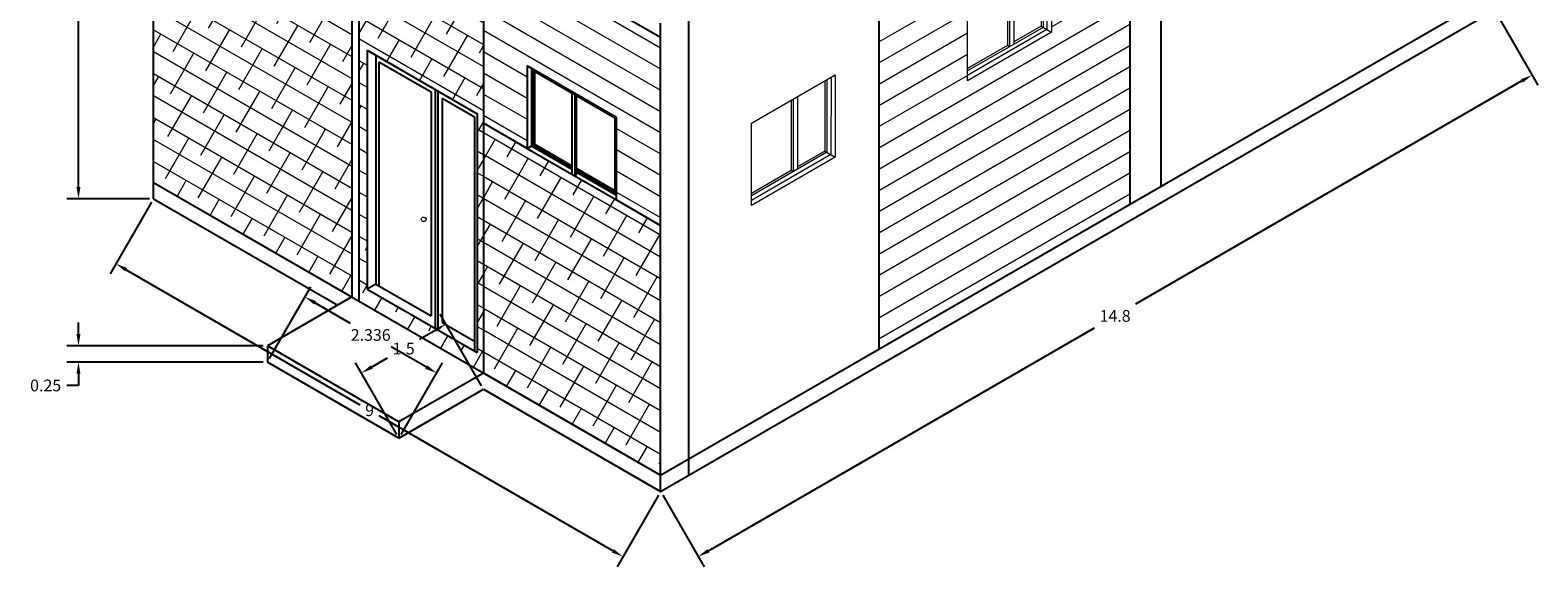
# Model space of a CAD drawing. Units: metres. Extents: x 14054 to 28215, y 4175 to 8383.
# Tile 1 of 6: x 14054 to 14077, y 4175 to 4183. Entities that reach past the tile are written whole.
import ezdxf

# ---------------------------------------------------------------- set-up
doc = ezdxf.new("R2010")
doc.units = ezdxf.units.M
for name, color, linetype, lineweight in [('A-ANNO-DIMS', 2, 'Continuous', 18), ('A-ELEV-ISOM', 7, 'Continuous', 25), ('A-FURN', 8, 'Continuous', 13), ('A-GLAZ', 4, 'Continuous', 18), ('A-WALL-PATT', 8, 'Continuous', 13)]:
    doc.layers.add(name, color=color, linetype=linetype, lineweight=lineweight)
doc.styles.get("Standard").update_dxf_attribs({"font": 'arial.ttf'})
doc.dimstyles.get("Standard").update_dxf_attribs({"dimtxt": 0.18, "dimasz": 0.18, "dimexe": 0.18, "dimexo": 0.0625, "dimgap": 0.09, "dimtad": 0, "dimtih": 1, "dimtoh": 1, "dimdec": 4, "dimzin": 0, "dimdsep": 46, "dimtxsty": 'Standard', "dimcen": 0.09, "dimadec": 0, "dimazin": 0, "dimtfac": 1, "dimtdec": 4, "dimtofl": 0, "dimtmove": 0, "dimatfit": 3, "dimfxl": 1, "dimtolj": 1, "dimtzin": 0, "dimarcsym": 0})

# ---------------------------------------------------------------- blocks, each defined once
blk = doc.blocks.new('WINDOW 1')
for p, q in [((14073.717, 4186.789), (14075.449, 4187.789)), ((14075.233, 4187.664), (14075.233, 4186.214)), ((14075.276, 4187.689), (14075.276, 4186.189)), ((14075.365, 4187.74), (14075.356, 4186.143)), ((14075.449, 4187.789), (14075.449, 4186.089)), ((14074.67, 4187.34), (14074.67, 4185.84)), ((14074.54, 4187.264), (14074.54, 4185.814)), ((14074.583, 4187.289), (14074.583, 4185.789)), ((14073.717, 4185.089), (14073.717, 4186.789)), ((14075.276, 4186.189), (14073.717, 4185.289)), ((14075.356, 4186.143), (14073.717, 4185.197)), ((14075.449, 4186.089), (14073.717, 4185.089)), ((14075.233, 4186.214), (14074.67, 4185.889)), ((14075.233, 4186.214), (14075.449, 4186.089)), ((14074.54, 4185.814), (14073.717, 4185.339)), ((14074.583, 4185.789), (14074.54, 4185.814))]:
    blk.add_line(p, q)
blk = doc.blocks.new('*D10')
at = {"layer": 'A-ANNO-DIMS', "color": 0, "lineweight": -2, "transparency": 16777216}
for p, q in [((14055.747, 4180.437), (14055.111, 4179.335)), ((14055.357, 4179.401), (14058.949, 4177.327)), ((14062.839, 4175.081), (14059.247, 4177.155)), ((14063.541, 4175.937), (14062.905, 4174.835))]:
    blk.add_line(p, q, dxfattribs=at)
at = {"layer": 'A-ANNO-DIMS', "color": 0, "transparency": 16777216}
for points in [[(14055.372, 4179.427), (14055.342, 4179.375), (14055.201, 4179.491)], [(14062.854, 4175.107), (14062.824, 4175.055), (14062.995, 4174.991)]]:
    blk.add_solid(points, dxfattribs=at)
at = {"layer": 'Defpoints', "color": 0, "transparency": 16777216}
for p in [(14055.778, 4180.491), (14055.201, 4179.491), (14063.573, 4175.991)]:
    blk.add_point(p, dxfattribs=at)
at = {"layer": 'A-ANNO-DIMS', "color": 0, "transparency": 16777216, "insert": (14059.098, 4177.241), "char_height": 0.18, "attachment_point": 5}
blk.add_mtext('\\A1;9', dxfattribs=at)
blk = doc.blocks.new('*D11')
at = {"layer": 'A-ANNO-DIMS', "color": 0, "lineweight": -2, "transparency": 16777216}
for p, q in [((14076.421, 4183.337), (14077.057, 4182.235)), ((14076.812, 4182.301), (14070.874, 4178.873)), ((14064.306, 4175.081), (14070.244, 4178.509)), ((14063.604, 4175.937), (14064.24, 4174.835))]:
    blk.add_line(p, q, dxfattribs=at)
at = {"layer": 'A-ANNO-DIMS', "color": 0, "transparency": 16777216}
for points in [[(14076.797, 4182.327), (14076.827, 4182.275), (14076.967, 4182.391)], [(14064.291, 4175.107), (14064.321, 4175.055), (14064.15, 4174.991)]]:
    blk.add_solid(points, dxfattribs=at)
at = {"layer": 'Defpoints', "color": 0, "transparency": 16777216}
for p in [(14076.39, 4183.391), (14063.573, 4175.991), (14064.15, 4174.991)]:
    blk.add_point(p, dxfattribs=at)
at = {"layer": 'A-ANNO-DIMS', "color": 0, "transparency": 16777216, "insert": (14070.559, 4178.691), "char_height": 0.18, "attachment_point": 5}
blk.add_mtext('\\A1;14.8', dxfattribs=at)
blk = doc.blocks.new('*D12')
at = {"layer": 'A-ANNO-DIMS', "color": 0, "lineweight": -2, "transparency": 16777216}
for p, q in [((14055.716, 4190.691), (14054.443, 4190.691)), ((14054.623, 4190.511), (14054.623, 4185.773)), ((14054.623, 4180.671), (14054.623, 4185.409)), ((14055.716, 4180.491), (14054.443, 4180.491))]:
    blk.add_line(p, q, dxfattribs=at)
at = {"layer": 'A-ANNO-DIMS', "color": 0, "transparency": 16777216}
for points in [[(14054.593, 4190.511), (14054.653, 4190.511), (14054.623, 4190.691)], [(14054.593, 4180.671), (14054.653, 4180.671), (14054.623, 4180.491)]]:
    blk.add_solid(points, dxfattribs=at)
at = {"layer": 'Defpoints', "color": 0, "transparency": 16777216}
for p in [(14054.623, 4190.691), (14055.778, 4190.691), (14055.778, 4180.491)]:
    blk.add_point(p, dxfattribs=at)
at = {"layer": 'A-ANNO-DIMS', "color": 0, "transparency": 16777216, "insert": (14054.623, 4185.591), "char_height": 0.18, "attachment_point": 5}
blk.add_mtext('\\A1;10.2', dxfattribs=at)
blk = doc.blocks.new('*D67')
at = {"layer": 'A-ANNO-DIMS', "color": 0, "lineweight": -2, "transparency": 16777216}
for p, q in [((14057.558, 4178.036), (14058.195, 4179.138)), ((14058.261, 4178.892), (14058.801, 4178.58)), ((14059.972, 4177.904), (14059.431, 4178.216)), ((14059.582, 4176.868), (14060.218, 4177.97))]:
    blk.add_line(p, q, dxfattribs=at)
at = {"layer": 'A-ANNO-DIMS', "color": 0, "transparency": 16777216}
for points in [[(14058.276, 4178.918), (14058.246, 4178.866), (14058.105, 4178.982)], [(14059.987, 4177.93), (14059.957, 4177.878), (14060.128, 4177.814)]]:
    blk.add_solid(points, dxfattribs=at)
at = {"layer": 'Defpoints', "color": 0, "transparency": 16777216}
for p in [(14057.527, 4177.982), (14060.128, 4177.814), (14059.55, 4176.814)]:
    blk.add_point(p, dxfattribs=at)
at = {"layer": 'A-ANNO-DIMS', "color": 0, "transparency": 16777216, "insert": (14059.116, 4178.398), "char_height": 0.18, "attachment_point": 5}
blk.add_mtext('\\A1;2.336', dxfattribs=at)
blk = doc.blocks.new('*D68')
at = {"layer": 'A-ANNO-DIMS', "color": 0, "lineweight": -2, "transparency": 16777216}
for p, q in [((14060.818, 4177.618), (14060.182, 4178.72)), ((14060.116, 4178.474), (14059.868, 4178.331)), ((14059.519, 4176.868), (14058.883, 4177.97)), ((14059.129, 4177.904), (14059.376, 4178.047))]:
    blk.add_line(p, q, dxfattribs=at)
at = {"layer": 'A-ANNO-DIMS', "color": 0, "transparency": 16777216}
for points in [[(14060.101, 4178.5), (14060.131, 4178.448), (14060.272, 4178.564)], [(14059.114, 4177.93), (14059.144, 4177.878), (14058.973, 4177.814)]]:
    blk.add_solid(points, dxfattribs=at)
at = {"layer": 'Defpoints', "color": 0, "transparency": 16777216}
for p in [(14060.272, 4178.564), (14060.849, 4177.564), (14059.55, 4176.814)]:
    blk.add_point(p, dxfattribs=at)
at = {"layer": 'A-ANNO-DIMS', "color": 0, "transparency": 16777216, "insert": (14059.622, 4178.189), "char_height": 0.18, "attachment_point": 5}
blk.add_mtext('\\A1;1.5', dxfattribs=at)
blk = doc.blocks.new('*D69')
at = {"layer": 'A-ANNO-DIMS', "color": 0, "lineweight": -2, "transparency": 16777216}
for p, q in [((14054.623, 4178.412), (14054.623, 4178.592)), ((14057.465, 4178.232), (14054.443, 4178.232)), ((14057.465, 4177.982), (14054.443, 4177.982)), ((14054.623, 4177.802), (14054.623, 4177.622)), ((14054.623, 4177.622), (14054.443, 4177.622))]:
    blk.add_line(p, q, dxfattribs=at)
at = {"layer": 'A-ANNO-DIMS', "color": 0, "transparency": 16777216}
for points in [[(14054.593, 4178.412), (14054.653, 4178.412), (14054.623, 4178.232)], [(14054.593, 4177.802), (14054.653, 4177.802), (14054.623, 4177.982)]]:
    blk.add_solid(points, dxfattribs=at)
at = {"layer": 'Defpoints', "color": 0, "transparency": 16777216}
for p in [(14057.527, 4178.232), (14054.623, 4177.982), (14057.527, 4177.982)]:
    blk.add_point(p, dxfattribs=at)
at = {"layer": 'A-ANNO-DIMS', "color": 0, "transparency": 16777216, "insert": (14054.119, 4177.622), "char_height": 0.18, "attachment_point": 5}
blk.add_mtext('\\A1;0.25', dxfattribs=at)

msp = doc.modelspace()

# ---------------------------------------------------------------- hatches: boundary and pattern name
at = {"layer": 'A-WALL-PATT'}
h = msp.add_hatch(dxfattribs=at)
h.set_pattern_fill('ANSI38', color=256, scale=0.092, angle=105)
h.paths.add_polyline_path([(14055.7785, 4187.4672), (14055.7785, 4180.7413), (14058.8262, 4178.9816), (14058.8262, 4185.7075)])
h.paths.add_polyline_path([(14058.0676, 4184.5273), (14058.0676, 4183.2595), (14056.6953, 4184.0519), (14056.6953, 4185.3196)], flags=16)
h.paths.add_polyline_path([(14056.7604, 4184.0895), (14056.7893, 4184.1061), (14056.7893, 4185.2436), (14058.0488, 4184.5164), (14058.0488, 4183.401), (14057.4455, 4183.7494), (14057.4455, 4183.6399), (14057.4272, 4183.6293), (14057.4272, 4184.8753), (14057.3815, 4184.9017), (14057.3815, 4183.7309)], flags=0)
h.paths.add_polyline_path([(14063.5727, 4180.0812), (14062.8942, 4180.4729), (14061.5218, 4181.2653), (14060.8587, 4181.6535), (14060.8401, 4177.8243), (14063.5727, 4176.2413)])
h.paths.add_polyline_path([(14060.8494, 4184.7636), (14060.9576, 4184.8261), (14058.9345, 4185.9941), (14058.9345, 4178.9191), (14060.8494, 4177.8136)])
h.paths.add_polyline_path([(14060.7529, 4181.7978), (14060.7529, 4181.7242), (14060.7529, 4178.127), (14059.0613, 4179.1036), (14059.0613, 4182.7744)], flags=16)
h.paths.add_polyline_path([(14059.2399, 4179.1538), (14059.2399, 4182.5977), (14060.0427, 4182.1342), (14060.0427, 4178.6903)], flags=0)
h.paths.add_polyline_path([(14060.215, 4182.0347), (14060.7096, 4181.7492), (14060.7096, 4178.3053), (14060.215, 4178.5908)], flags=0)
edge = h.paths.add_edge_path(flags=0)
edge.add_ellipse((14059.9307, 4180.1763), major_axis=(-0.0333, 0.0192), ratio=0.8810932, start_angle=0, end_angle=360)
h = msp.add_hatch(dxfattribs=at)
h.set_pattern_fill('ANSI31', color=256, scale=0.089, angle=165)
h.paths.add_polyline_path([(14070.7875, 4187.3567), (14066.9286, 4185.1288), (14066.9286, 4178.1788), (14070.7875, 4180.4067)])
h.paths.add_polyline_path([(14069.5808, 4184.3152), (14069.5808, 4183.05), (14068.2917, 4182.3057), (14068.2917, 4183.5709)], flags=16)
h.paths.add_polyline_path([(14069.4519, 4183.1244), (14069.0007, 4182.8639), (14069.0007, 4182.9011), (14069.4197, 4183.143)], flags=0)
h = msp.add_hatch(dxfattribs=at)
h.set_pattern_fill('ANSI31', color=256, scale=0.089, angle=105)
h.paths.add_polyline_path([(14063.5727, 4182.9672), (14060.8494, 4184.5395), (14060.8494, 4181.6535), (14061.5218, 4181.2653), (14061.5218, 4182.533), (14062.8942, 4181.7407), (14062.8942, 4180.4729), (14063.5727, 4180.0812)])

# ---------------------------------------------------------------- linework, layer by layer
at = {"layer": 'A-ELEV-ISOM'}
for p, q in [((14070.7875, 4190.3575), (14070.7875, 4180.4067)), ((14055.7785, 4180.4913), (14055.7785, 4187.6913)), ((14071.2638, 4187.6317), (14071.2638, 4180.6817)), ((14058.9345, 4185.9941), (14058.9345, 4178.9191)), ((14058.8262, 4185.9316), (14058.8262, 4178.9816)), ((14066.9286, 4185.1288), (14066.9286, 4178.1788)), ((14060.8494, 4184.7636), (14060.8494, 4177.8136)), ((14063.5727, 4182.9672), (14060.8494, 4184.5395)), ((14063.5727, 4176.2413), (14076.3899, 4183.6413)), ((14064.0057, 4176.2413), (14064.0057, 4183.4413)), ((14063.5727, 4175.9913), (14076.3899, 4183.3913)), ((14063.5727, 4175.9913), (14063.5727, 4183.1913)), ((14059.0613, 4182.7744), (14060.7529, 4181.7978)), ((14059.0613, 4182.7744), (14059.0613, 4179.1036)), ((14059.194, 4182.6978), (14059.194, 4179.1803)), ((14059.2399, 4182.5977), (14060.0427, 4182.1342)), ((14059.2399, 4182.5977), (14059.2399, 4179.1538)), ((14062.8942, 4181.7407), (14061.5218, 4182.533)), ((14061.5218, 4182.533), (14061.5218, 4181.2653)), ((14061.5869, 4182.4954), (14061.5869, 4181.3029)), ((14061.6158, 4182.457), (14061.6158, 4181.3195)), ((14062.8754, 4181.7298), (14061.6158, 4182.457)), ((14061.635, 4182.446), (14061.635, 4181.3306)), ((14060.0427, 4182.1342), (14060.0427, 4178.6903)), ((14060.1077, 4182.1703), (14060.1077, 4178.4995)), ((14060.1465, 4182.1479), (14060.1465, 4178.4771)), ((14062.208, 4182.1151), (14062.208, 4180.8691)), ((14062.2537, 4182.0887), (14062.2537, 4180.8427)), ((14062.272, 4182.0781), (14062.272, 4180.8533)), ((14060.215, 4182.0347), (14060.215, 4178.5908)), ((14060.215, 4182.0347), (14060.7096, 4181.7492)), ((14060.7096, 4181.7492), (14060.7096, 4178.152)), ((14060.7529, 4181.7978), (14060.7529, 4181.7242)), ((14060.7529, 4181.7242), (14060.7529, 4178.127)), ((14061.5218, 4181.2653), (14060.8494, 4181.6535)), ((14062.8754, 4180.6144), (14062.8754, 4181.7298)), ((14062.8942, 4180.4729), (14062.8942, 4181.7407)), ((14061.5218, 4181.2653), (14061.635, 4181.3306)), ((14061.5218, 4181.2653), (14062.8942, 4180.4729)), ((14061.5869, 4181.3029), (14062.208, 4180.9443)), ((14061.6158, 4181.3195), (14062.208, 4180.9777)), ((14061.635, 4181.3306), (14062.208, 4180.9997)), ((14062.272, 4180.9628), (14062.8754, 4180.6144)), ((14062.272, 4180.9407), (14062.8942, 4180.5815)), ((14062.272, 4180.9073), (14062.8942, 4180.5481)), ((14055.7785, 4180.7413), (14063.5727, 4176.2413)), ((14055.7785, 4180.7413), (14058.8262, 4178.9816)), ((14062.2537, 4180.8427), (14062.272, 4180.8533)), ((14055.7785, 4180.4913), (14058.6097, 4178.8566)), ((14062.8942, 4180.4729), (14063.5727, 4180.0812)), ((14059.194, 4179.1803), (14059.0613, 4179.1036)), ((14059.0613, 4179.1036), (14060.7529, 4178.127)), ((14059.194, 4179.1803), (14060.0427, 4178.6903)), ((14058.8262, 4178.9816), (14057.5272, 4178.2316)), ((14060.215, 4178.5908), (14060.7096, 4178.3053)), ((14059.5503, 4177.0636), (14057.5272, 4178.2316)), ((14057.5272, 4178.2316), (14057.5272, 4177.9816)), ((14059.5503, 4176.8136), (14057.5272, 4177.9816)), ((14060.8494, 4177.8136), (14059.5503, 4177.0636)), ((14060.8308, 4177.8243), (14063.5727, 4176.2413)), ((14059.5503, 4176.8136), (14060.8494, 4177.5636)), ((14060.8494, 4177.5636), (14063.5727, 4175.9913)), ((14059.5503, 4177.0636), (14059.5503, 4176.8136))]:
    msp.add_line(p, q, dxfattribs=at)
at = {"layer": 'A-FURN'}
msp.add_ellipse((14059.9307, 4180.1763), major_axis=(-0.0333, 0.0192), ratio=0.8810932, start_param=-3.141592653589793, end_param=3.141592653589793, dxfattribs=at)

# ---------------------------------------------------------------- block references
at = {"layer": 'A-GLAZ', "xscale": 0.7442386112486127, "yscale": 0.7442386112486127, "zscale": 0.7442386112486127}
for p in [(3594.088, 1067.601), (3590.7636, 1065.6817)]:
    msp.add_blockref('WINDOW 1', p, dxfattribs=at)

# ---------------------------------------------------------------- dimensions: what is measured, and where the dimension line sits
at = {"layer": 'A-ANNO-DIMS'}
for base, p1, p2, angle, override, picture, middle in [((14054.6235, 4190.6913), (14055.7785, 4180.4913), (14055.7785, 4190.6913), 90, {"dimdec": 1, "dimlfac": 1, "dimrnd": 0, "dimzin": 0, "dimdsep": 46, "dimlunit": 2}, '*D12', (14054.6235, 4185.5913)), ((14064.1502, 4174.991), (14076.3899, 4183.3913), (14063.5727, 4175.9913), 210, {"dimdec": 1, "dimlfac": 1, "dimrnd": 0, "dimzin": 0, "dimdsep": 46, "dimlunit": 2}, '*D11', (14070.5588, 4178.691)), ((14055.201, 4179.491), (14063.5727, 4175.9913), (14055.7785, 4180.4913), 150, {"dimdec": 0, "dimlfac": 1, "dimrnd": 0, "dimzin": 0, "dimdsep": 46, "dimlunit": 2}, '*D10', (14059.0981, 4177.241)), ((14060.1278, 4177.8138), (14057.5272, 4177.9816), (14059.5503, 4176.8136), 330, {"dimdec": 3, "dimlfac": 1, "dimrnd": 0, "dimzin": 0, "dimdsep": 46, "dimlunit": 2}, '*D67', (14059.1163, 4178.3979)), ((14054.6235, 4177.9816), (14057.5272, 4178.2316), (14057.5272, 4177.9816), 90, {"dimdec": 2, "dimlfac": 1, "dimrnd": 0, "dimzin": 0, "dimdsep": 46, "dimlunit": 2}, '*D69', (14054.119, 4177.6216)), ((14060.2719, 4178.5638), (14059.5503, 4176.8136), (14060.8494, 4177.5636), 30, {"dimdec": 1, "dimlfac": 1, "dimrnd": 0, "dimzin": 0, "dimdsep": 46, "dimlunit": 2}, '*D68', (14059.6224, 4178.1888))]:
    dim = msp.add_linear_dim(base=base, p1=p1, p2=p2, angle=angle, dimstyle='Standard', override=override, dxfattribs=at)
    dim.commit()
    dim.dimension.update_dxf_attribs({"geometry": picture, "text_midpoint": middle})

doc.saveas('drawing.dxf')
